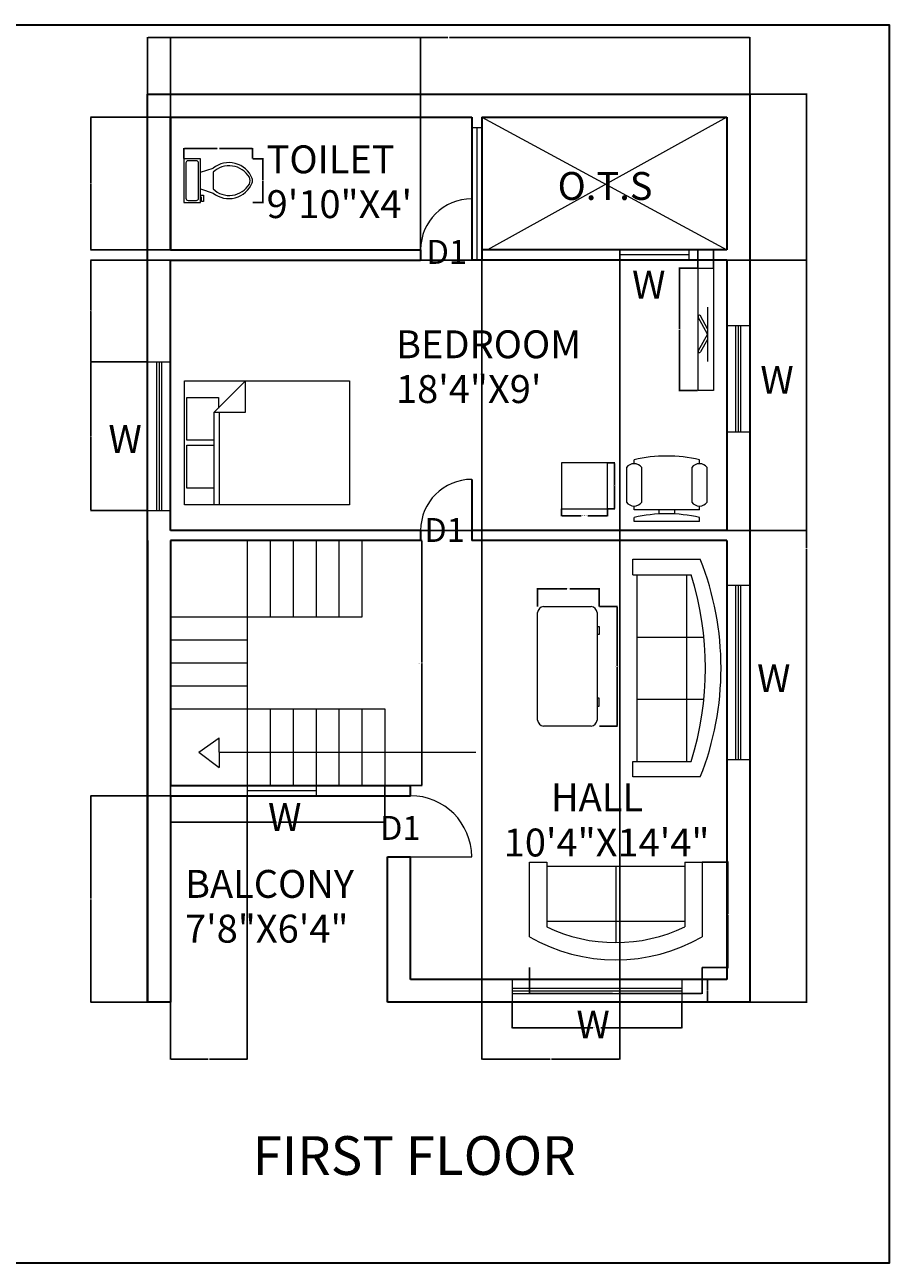
# Model space of a CAD drawing. Units: feet. Extents: x 38163 to 38841, y 65807 to 66292.
# Tile 3 of 3: x 38502 to 38841, y 65807 to 66292. Entities that reach past the tile are written whole.
import ezdxf

# ---------------------------------------------------------------- set-up
doc = ezdxf.new("R2010")
doc.units = ezdxf.units.FT
for name, color, linetype, lineweight in [('A-ANNO-DIMS', 2, 'Continuous', 18), ('A-ANNO-SYMB', 7, 'Continuous', 13), ('A-ANNO-TEXT', 7, 'Continuous', 18), ('A-ANNO-TITL', 7, 'Continuous', 25), ('A-ANNO-TTLB', 7, 'Continuous', 35), ('A-AREA-IDEN', 7, 'Continuous', 18), ('A-DOOR', 4, 'Continuous', 18), ('A-FLOR-FIXT', 9, 'Continuous', 18), ('A-FLOR-OPEN', 8, 'Continuous', 13), ('A-FLOR-STRS', 7, 'Continuous', 18), ('A-FURN', 8, 'Continuous', 18), ('A-GLAZ', 4, 'Continuous', 13), ('A-WALL', 7, 'Continuous', 35)]:
    doc.layers.add(name, color=color, linetype=linetype, lineweight=lineweight)
doc.styles.get("Standard").update_dxf_attribs({"font": 'arial.ttf'})
doc.dimstyles.get("Standard").update_dxf_attribs({"dimtxt": 0.18, "dimasz": 0.18, "dimexe": 0.18, "dimexo": 0.0625, "dimgap": 0.09, "dimtad": 0, "dimtih": 1, "dimtoh": 1, "dimdec": 4, "dimzin": 0, "dimdsep": 46, "dimtxsty": 'Standard', "dimcen": 0.09, "dimadec": 0, "dimazin": 0, "dimtfac": 1, "dimtdec": 4, "dimtofl": 0, "dimtmove": 0, "dimatfit": 3, "dimfxl": 1, "dimtolj": 1, "dimtzin": 0, "dimarcsym": 0})

# ---------------------------------------------------------------- blocks, each defined once
blk = doc.blocks.new('Toilet - top')
for p, q in [((9.5, -6), (9.5, -2)), ((-10, -8.5), (-8, -8.5)), ((-10, -9.5), (-10, -8.5)), ((-7, -9.5), (-10, -9.5)), ((-8, -8.5), (-8, -8)), ((-7, -8), (-7, -9.5)), ((-4, -8), (-6, -14)), ((4, -8), (6, -14)), ((4, -14), (-4, -14))]:
    blk.add_line(p, q)
blk.add_lwpolyline([(10.5, -8), (10.5, 0), (-10.5, 0), (-10.5, -8)], close=True)
for points in [[(-9.5, -2), (-9.5, -6)], [(8.5, -1), (-8.5, -1)], [(-8.5, -7), (8.5, -7)]]:
    blk.add_lwpolyline(points)
for centre, radius, start, end in [((-8.62, -1.88), 0.884, 81.8699, 188.1301), ((8.62, -1.88), 0.884, 351.8699, 98.1301), ((-8.62, -6.12), 0.884, 171.8699, 278.1301), ((8.62, -6.12), 0.884, 261.8699, 8.1301), ((3.52, -21.58), 12.17, 141.46911, 247.97143), ((4.2, -21.82), 11.33, 136.36773, 238.94682), ((-3.52, -21.58), 12.17, 292.02843, 38.53071), ((-4.2, -21.82), 11.33, 301.05301, 43.63209), ((0, -27.88), 4, 245.73182, 294.26817), ((0, -29), 4, 254.86053, 285.13947)]:
    blk.add_arc(centre, radius, start, end)
blk = doc.blocks.new('Bed - Queen')
for p, q in [((0, -80.00003), (0, 0)), ((0, 0), (59.99999, 0)), ((59.99999, 0), (59.99999, -80.00003)), ((7.99999, -1.2), (28.79998, -1.2)), ((7.99999, -14.4), (7.99999, -1.2)), ((28.79998, -1.2), (28.79998, -14.4)), ((31.19999, -1.2), (51.99999, -1.2)), ((31.19999, -14.4), (31.19999, -1.2)), ((51.99999, -1.2), (51.99999, -16.4)), ((0, -14.4), (44.8, -14.4)), ((44.8, -16.8), (0, -16.8)), ((59.99999, -29.6), (44.8, -14.4)), ((44.8, -14.4), (44.8, -29.6)), ((51.99999, -16.4), (46.79936, -16.4)), ((44.8, -29.6), (59.99999, -29.6)), ((59.99999, -80.00003), (0, -80.00003))]:
    blk.add_line(p, q)
blk = doc.blocks.new('Chair - Desk')
for p, q in [((-8.5, 0), (-8.5, -1)), ((-8.5, 0), (8.5, 0)), ((8.5, 0), (8.5, -1)), ((-8.5, -3), (-8.5, -4)), ((-8.5, -3), (8.5, -3)), ((-2, -3), (-2, -1.9355)), ((2, -1.9576), (2, -3)), ((8.5, -3), (8.5, -4)), ((-10.5, -5), (-10.5, -14)), ((-6.5, -14), (-6.5, -5)), ((6.5, -5), (6.5, -14)), ((10.5, -14), (10.5, -5)), ((-8.5, -15), (-8.5, -16)), ((8.5, -15), (8.5, -16))]:
    blk.add_line(p, q)
for centre, radius, start, end in [((0, 34.625), 36.625, 256.5803, 283.4197), ((-8.5, -6.5), 2.5, 36.8699, 143.1301), ((8.5, -6.5), 2.5, 36.8699, 143.1301), ((-8.5, -12.5), 2.5, 216.8699, 323.1301), ((0, 19.625), 36.625, 256.5803, 283.4197), ((8.5, -12.5), 2.5, 216.8699, 323.1301)]:
    blk.add_arc(centre, radius, start, end)
blk = doc.blocks.new('Desk - 30 x 60 in.')
for p, q in [((-26.999995, 0), (26.999995, 0)), ((-29.999995, -27), (-29.999995, -3)), ((29.999995, -3), (29.999995, -27)), ((26.999995, -30), (-26.999995, -30)), ((-20.000005, -30), (-20.000005, -31)), ((-20.000005, -31), (-16.000005, -31)), ((-16.000005, -31), (-16.000005, -30)), ((15.999995, -31), (15.999995, -30)), ((19.999995, -31), (15.999995, -31)), ((19.999995, -30), (19.999995, -31))]:
    blk.add_line(p, q)
for centre, start, end in [((-26.499995, -3.5), 98.1301, 171.8699), ((26.499995, -3.5), 8.130102, 81.8699), ((-26.499995, -26.5), 188.1301, 261.8699), ((26.499995, -26.5), 278.1301, 351.8699)]:
    blk.add_arc(centre, 3.535534, start, end)
blk = doc.blocks.new('Sofa - Roundback 7 ft.')
for p, q in [((-12.00002, -32.4421), (-12.00003, -6.5971)), ((11.99997, -32.4421), (11.99998, -6.5971)), ((-36.000027, -34), (-36.000027, -11.4696)), ((-35.999844, -13.3819), (35.9998, -13.3819)), ((35.99998, -34), (35.99998, -11.4696)), ((-36.000027, -32.4421), (35.99998, -32.4421))]:
    blk.add_line(p, q)
for points in [[(-36.000027, -34), (-42.000027, -34), (-42.000027, -8)], [(41.99998, -8), (41.99998, -34), (35.99998, -34)]]:
    blk.add_lwpolyline(points)
for centre, radius, start, end in [((0, -114.25), 114.25, 68.43141, 111.5686), ((-0.00001, -127.1968), 121.1968, 72.72033, 107.2797)]:
    blk.add_arc(centre, radius, start, end)
blk = doc.blocks.new('Sofa - Roundback Loveseat 5 ft.')
for p, q in [((0, -32.44198), (0, -5.99998)), ((-24, -33.99998), (-24, -11.46958)), ((24.00004, -33.99998), (24.00004, -11.46958)), ((-23.9998, -13.38178), (23.99986, -13.38178)), ((-24, -32.44198), (24.00004, -32.44198))]:
    blk.add_line(p, q)
for points in [[(-24, -33.99998), (-30, -33.99998), (-30, -7.99998)], [(30.00004, -7.99998), (30.00004, -33.99998), (24.00004, -33.99998)]]:
    blk.add_lwpolyline(points)
for centre, radius, start, end in [((0, -60.24998), 60.24998, 60.13715, 119.8628), ((0, -61.38438), 55.38444, 64.32083, 115.6792)]:
    blk.add_arc(centre, radius, start, end)
blk = doc.blocks.new('DOOR-SWING-24')
blk.add_line((0, 0), (24, 0))
blk.add_arc((0, 0), 24, 0, 90)
blk = doc.blocks.new('DOOR-SWING-20')
blk.add_line((20, 0), (20, 20))
blk.add_arc((20, 0), 20, 90, 180)
blk = doc.blocks.new('STAIR-HALF-TURN')
for p, q in [((30, 96), (30, 0)), ((39, 96), (39, 66)), ((48, 96), (48, 66)), ((57, 96), (57, 66)), ((66, 96), (66, 66)), ((75, 96), (75, 66)), ((75, 66), (0, 66)), ((30, 57), (0, 57)), ((30, 48), (0, 48)), ((30, 39), (0, 39)), ((0, 30), (84, 30)), ((39, 30), (39, 0)), ((48, 30), (48, 0)), ((57, 30), (57, 0)), ((66, 30), (66, 0)), ((75, 30), (75, 0)), ((84, 30), (84, 0))]:
    blk.add_line(p, q)
blk = doc.blocks.new('TABLE-SQUARE')
for p, q in [((18, 18), (0, 18)), ((0, 18), (0, 0)), ((18, 0), (18, 18)), ((0, 0), (18, 0))]:
    blk.add_line(p, q)
blk = doc.blocks.new('TV-CONSOLE')
for p, q in [((0.06, 48), (6.06, 48)), ((0.06, 0), (0.06, 48)), ((6.06, 48), (6.06, 0)), ((3.68, 24.21), (0.94, 29.3)), ((3.68, 32.75), (3.68, 11.44)), ((3.68, 22.09), (0.06, 28.83)), ((3.68, 22.09), (0.06, 15.67)), ((3.68, 20.06), (0.93, 15.18)), ((6.06, 0), (0.06, 0))]:
    blk.add_line(p, q)
for centre, start, end in [((0.5, 29.07), 28.2522, 208.2522), ((0.5, 15.42), 150.6168, 330.6168)]:
    blk.add_arc(centre, 0.5, start, end)
blk = doc.blocks.new('WIN-FRONT-HALL')
for p, q in [((0, 9), (0, 0)), ((0, 5.5), (66.57, 5.5)), ((66.57, 9), (66.57, 0)), ((0, 4.5), (66.57, 4.5)), ((0, 3.5), (66.57, 3.5))]:
    blk.add_line(p, q)
blk = doc.blocks.new('WIN-SIDE-HALL')
for p, q in [((0, 68.38), (9, 68.38)), ((3.5, 68.38), (3.5, 0)), ((4.5, 68.38), (4.5, 0)), ((5.5, 68.38), (5.5, 0)), ((0, 0), (9, 0))]:
    blk.add_line(p, q)
blk = doc.blocks.new('WIN-SIDE-REAR')
for p, q in [((0, 41.67), (9, 41.67)), ((3.5, 41.67), (3.5, 0)), ((4.5, 41.67), (4.5, 0)), ((5.5, 41.67), (5.5, 0)), ((0, 0), (9, 0))]:
    blk.add_line(p, q)
blk = doc.blocks.new('WIN-STAIR')
for p, q in [((0, 4), (0, 0)), ((0, 2), (27, 2)), ((27, 4), (27, 0))]:
    blk.add_line(p, q)
blk = doc.blocks.new('WIN-LIGHTWELL')
for p, q in [((0, 0), (0, 4)), ((0, 2), (27.16, 2)), ((27.16, 0), (27.16, 4))]:
    blk.add_line(p, q)
blk = doc.blocks.new('LIGHTWELL-CROSS')
for p, q in [((0, 52), (96, 0)), ((96, 52), (2.18, 0))]:
    blk.add_line(p, q)
blk = doc.blocks.new('STAIR-ARROWHEAD')
for p, q in [((0, 6), (8, 11.63)), ((8, 6), (8, 11.63)), ((0, 6), (8, 0)), ((8, 6), (8, 0)), ((8, 0), (8, 0))]:
    blk.add_line(p, q)
blk = doc.blocks.new('*D29')
at = {"layer": 'A-ANNO-DIMS', "color": 0, "lineweight": -2, "transparency": 16777216}
for p, q in [((38727.19, 66064.14), (38734.33, 66064.14)), ((38734.15, 66063.96), (38734.15, 66040.91)), ((38734.15, 66017.51), (38734.15, 66040.55)), ((38727.19, 66017.33), (38734.33, 66017.33))]:
    blk.add_line(p, q, dxfattribs=at)
at = {"layer": 'A-ANNO-DIMS', "color": 0, "transparency": 16777216}
for points in [[(38734.12, 66063.96), (38734.18, 66063.96), (38734.15, 66064.14)], [(38734.12, 66017.51), (38734.18, 66017.51), (38734.15, 66017.33)]]:
    blk.add_solid(points, dxfattribs=at)
at = {"layer": 'Defpoints', "color": 0, "transparency": 16777216}
for p in [(38727.13, 66064.14), (38734.15, 66064.14), (38727.13, 66017.33)]:
    blk.add_point(p, dxfattribs=at)
at = {"layer": 'A-ANNO-DIMS', "color": 0, "transparency": 16777216, "insert": (38734.15, 66040.73), "char_height": 0.18, "attachment_point": 5}
blk.add_mtext('\\A1;DESK 47 TYP.', dxfattribs=at)
blk = doc.blocks.new('*D30')
at = {"layer": 'A-ANNO-DIMS', "color": 0, "lineweight": -2, "transparency": 16777216}
for p, q in [((38702.94, 66064.2), (38702.94, 66071.34)), ((38703.12, 66071.16), (38714.51, 66071.16)), ((38726.95, 66071.16), (38715.57, 66071.16)), ((38727.13, 66064.2), (38727.13, 66071.34))]:
    blk.add_line(p, q, dxfattribs=at)
at = {"layer": 'A-ANNO-DIMS', "color": 0, "transparency": 16777216}
for points in [[(38703.12, 66071.19), (38703.12, 66071.13), (38702.94, 66071.16)], [(38726.95, 66071.19), (38726.95, 66071.13), (38727.13, 66071.16)]]:
    blk.add_solid(points, dxfattribs=at)
at = {"layer": 'Defpoints', "color": 0, "transparency": 16777216}
for p in [(38702.94, 66071.16), (38702.94, 66064.14), (38727.13, 66064.14)]:
    blk.add_point(p, dxfattribs=at)
at = {"layer": 'A-ANNO-DIMS', "color": 0, "transparency": 16777216, "insert": (38715.04, 66071.16), "char_height": 0.18, "attachment_point": 5}
blk.add_mtext('\\A1;24 TYP.', dxfattribs=at)
blk = doc.blocks.new('*D33')
at = {"layer": 'A-ANNO-DIMS', "color": 0, "lineweight": -2, "transparency": 16777216}
for p, q in [((38699.8, 65922.6), (38699.8, 65912.34)), ((38767.45, 65922.6), (38767.45, 65912.34)), ((38699.98, 65912.52), (38732.4, 65912.52)), ((38767.27, 65912.52), (38734.85, 65912.52))]:
    blk.add_line(p, q, dxfattribs=at)
at = {"layer": 'A-ANNO-DIMS', "color": 0, "transparency": 16777216}
for points in [[(38699.98, 65912.55), (38699.98, 65912.49), (38699.8, 65912.52)], [(38767.27, 65912.55), (38767.27, 65912.49), (38767.45, 65912.52)]]:
    blk.add_solid(points, dxfattribs=at)
at = {"layer": 'Defpoints', "color": 0, "transparency": 16777216}
for p in [(38699.8, 65922.66), (38767.45, 65922.66), (38699.8, 65912.52)]:
    blk.add_point(p, dxfattribs=at)
at = {"layer": 'A-ANNO-DIMS', "color": 0, "transparency": 16777216, "insert": (38733.63, 65912.52), "char_height": 0.18, "attachment_point": 5}
blk.add_mtext('\\A1;LOVESEAT 68 TYP.', dxfattribs=at)
blk = doc.blocks.new('*D34')
at = {"layer": 'A-ANNO-DIMS', "color": 0, "lineweight": -2, "transparency": 16777216}
for p, q in [((38767.51, 65964.01), (38777.78, 65964.01)), ((38777.6, 65963.83), (38777.6, 65943.52)), ((38777.6, 65922.84), (38777.6, 65943.16)), ((38767.51, 65922.66), (38777.78, 65922.66))]:
    blk.add_line(p, q, dxfattribs=at)
at = {"layer": 'A-ANNO-DIMS', "color": 0, "transparency": 16777216}
for points in [[(38777.57, 65963.83), (38777.63, 65963.83), (38777.6, 65964.01)], [(38777.57, 65922.84), (38777.63, 65922.84), (38777.6, 65922.66)]]:
    blk.add_solid(points, dxfattribs=at)
at = {"layer": 'Defpoints', "color": 0, "transparency": 16777216}
for p in [(38767.45, 65964.01), (38767.45, 65922.66), (38777.6, 65922.66)]:
    blk.add_point(p, dxfattribs=at)
at = {"layer": 'A-ANNO-DIMS', "color": 0, "transparency": 16777216, "insert": (38777.6, 65943.34), "char_height": 0.18, "attachment_point": 5}
blk.add_mtext('\\A1;41 TYP.', dxfattribs=at)
blk = doc.blocks.new('*D35')
at = {"layer": 'A-ANNO-DIMS', "color": 0, "lineweight": -2, "transparency": 16777216}
for p, q in [((38643.22, 66090.01), (38657.74, 66090.01)), ((38657.56, 66089.83), (38657.56, 66042.2)), ((38657.56, 65994.19), (38657.56, 66041.83)), ((38643.22, 65994.01), (38657.74, 65994.01))]:
    blk.add_line(p, q, dxfattribs=at)
at = {"layer": 'A-ANNO-DIMS', "color": 0, "transparency": 16777216}
for points in [[(38657.53, 66089.83), (38657.59, 66089.83), (38657.56, 66090.01)], [(38657.53, 65994.19), (38657.59, 65994.19), (38657.56, 65994.01)]]:
    blk.add_solid(points, dxfattribs=at)
at = {"layer": 'Defpoints', "color": 0, "transparency": 16777216}
for p in [(38643.16, 66090.01), (38657.56, 66090.01), (38643.16, 65994.01)]:
    blk.add_point(p, dxfattribs=at)
at = {"layer": 'A-ANNO-DIMS', "color": 0, "transparency": 16777216, "insert": (38657.56, 66042.01), "char_height": 0.18, "attachment_point": 5}
blk.add_mtext('\\A1;HALF-TURN STAIR 96 TYP.', dxfattribs=at)
blk = doc.blocks.new('*D36')
at = {"layer": 'A-ANNO-DIMS', "color": 0, "lineweight": -2, "transparency": 16777216}
for p, q in [((38559.16, 65993.95), (38559.16, 65979.43)), ((38643.16, 65993.95), (38643.16, 65979.43)), ((38559.34, 65979.61), (38600.63, 65979.61)), ((38642.98, 65979.61), (38601.69, 65979.61))]:
    blk.add_line(p, q, dxfattribs=at)
at = {"layer": 'A-ANNO-DIMS', "color": 0, "transparency": 16777216}
for points in [[(38559.34, 65979.64), (38559.34, 65979.58), (38559.16, 65979.61)], [(38642.98, 65979.64), (38642.98, 65979.58), (38643.16, 65979.61)]]:
    blk.add_solid(points, dxfattribs=at)
at = {"layer": 'Defpoints', "color": 0, "transparency": 16777216}
for p in [(38559.16, 65994.01), (38643.16, 65994.01), (38643.16, 65979.61)]:
    blk.add_point(p, dxfattribs=at)
at = {"layer": 'A-ANNO-DIMS', "color": 0, "transparency": 16777216, "insert": (38601.16, 65979.61), "char_height": 0.18, "attachment_point": 5}
blk.add_mtext('\\A1;84 TYP.', dxfattribs=at)
blk = doc.blocks.new('*D37')
at = {"layer": 'A-ANNO-DIMS', "color": 0, "lineweight": -2, "transparency": 16777216}
for p, q in [((38712.38, 66102.41), (38712.38, 66099.6)), ((38730.38, 66102.41), (38730.38, 66099.6)), ((38712.56, 66099.78), (38720.09, 66099.78)), ((38730.2, 66099.78), (38722.67, 66099.78))]:
    blk.add_line(p, q, dxfattribs=at)
at = {"layer": 'A-ANNO-DIMS', "color": 0, "transparency": 16777216}
for points in [[(38712.56, 66099.81), (38712.56, 66099.75), (38712.38, 66099.78)], [(38730.2, 66099.81), (38730.2, 66099.75), (38730.38, 66099.78)]]:
    blk.add_solid(points, dxfattribs=at)
at = {"layer": 'Defpoints', "color": 0, "transparency": 16777216}
for p in [(38712.38, 66102.48), (38730.38, 66102.48), (38730.38, 66099.78)]:
    blk.add_point(p, dxfattribs=at)
at = {"layer": 'A-ANNO-DIMS', "color": 0, "transparency": 16777216, "insert": (38721.38, 66099.78), "char_height": 0.18, "attachment_point": 5}
blk.add_mtext('\\A1;SIDE TABLE 18 TYP.', dxfattribs=at)
blk = doc.blocks.new('*D38')
at = {"layer": 'A-ANNO-DIMS', "color": 0, "lineweight": -2, "transparency": 16777216}
for p, q in [((38730.44, 66120.48), (38733.26, 66120.48)), ((38733.08, 66120.3), (38733.08, 66111.66)), ((38733.08, 66102.66), (38733.08, 66111.3)), ((38730.44, 66102.48), (38733.26, 66102.48))]:
    blk.add_line(p, q, dxfattribs=at)
at = {"layer": 'A-ANNO-DIMS', "color": 0, "transparency": 16777216}
for points in [[(38733.05, 66120.3), (38733.11, 66120.3), (38733.08, 66120.48)], [(38733.05, 66102.66), (38733.11, 66102.66), (38733.08, 66102.48)]]:
    blk.add_solid(points, dxfattribs=at)
at = {"layer": 'Defpoints', "color": 0, "transparency": 16777216}
for p in [(38730.38, 66120.48), (38733.08, 66120.48), (38730.38, 66102.48)]:
    blk.add_point(p, dxfattribs=at)
at = {"layer": 'A-ANNO-DIMS', "color": 0, "transparency": 16777216, "insert": (38733.08, 66111.48), "char_height": 0.18, "attachment_point": 5}
blk.add_mtext('\\A1;18 TYP.', dxfattribs=at)
blk = doc.blocks.new('*D39')
at = {"layer": 'A-ANNO-DIMS', "color": 0, "lineweight": -2, "transparency": 16777216}
for p, q in [((38765.71, 66196.8), (38758.39, 66196.8)), ((38758.57, 66196.62), (38758.57, 66172.99)), ((38758.57, 66148.98), (38758.57, 66172.62)), ((38765.71, 66148.8), (38758.39, 66148.8))]:
    blk.add_line(p, q, dxfattribs=at)
at = {"layer": 'A-ANNO-DIMS', "color": 0, "transparency": 16777216}
for points in [[(38758.54, 66196.62), (38758.6, 66196.62), (38758.57, 66196.8)], [(38758.54, 66148.98), (38758.6, 66148.98), (38758.57, 66148.8)]]:
    blk.add_solid(points, dxfattribs=at)
at = {"layer": 'Defpoints', "color": 0, "transparency": 16777216}
for p in [(38758.57, 66196.8), (38765.77, 66196.8), (38765.77, 66148.8)]:
    blk.add_point(p, dxfattribs=at)
at = {"layer": 'A-ANNO-DIMS', "color": 0, "transparency": 16777216, "insert": (38758.57, 66172.8), "char_height": 0.18, "attachment_point": 5}
blk.add_mtext('\\A1;TV CONSOLE 48 TYP.', dxfattribs=at)
blk = doc.blocks.new('*D40')
at = {"layer": 'A-ANNO-DIMS', "color": 0, "lineweight": -2, "transparency": 16777216}
for p, q in [((38765.77, 66196.87), (38765.77, 66204.18)), ((38765.95, 66204), (38768.38, 66204)), ((38771.72, 66204), (38769.29, 66204)), ((38771.9, 66196.87), (38771.9, 66204.18))]:
    blk.add_line(p, q, dxfattribs=at)
at = {"layer": 'A-ANNO-DIMS', "color": 0, "transparency": 16777216}
for points in [[(38765.95, 66204.03), (38765.95, 66203.97), (38765.77, 66204)], [(38771.72, 66204.03), (38771.72, 66203.97), (38771.9, 66204)]]:
    blk.add_solid(points, dxfattribs=at)
at = {"layer": 'Defpoints', "color": 0, "transparency": 16777216}
for p in [(38771.9, 66204), (38765.77, 66196.8), (38771.9, 66196.8)]:
    blk.add_point(p, dxfattribs=at)
at = {"layer": 'A-ANNO-DIMS', "color": 0, "transparency": 16777216, "insert": (38768.84, 66204), "char_height": 0.18, "attachment_point": 5}
blk.add_mtext('\\A1;6 TYP.', dxfattribs=at)
blk = doc.blocks.new('*D41')
at = {"layer": 'A-ANNO-DIMS', "color": 0, "lineweight": -2, "transparency": 16777216}
for p, q in [((38692.96, 65908.95), (38692.96, 65898.85)), ((38759.53, 65908.95), (38759.53, 65898.85)), ((38693.14, 65899.03), (38724.67, 65899.03)), ((38759.35, 65899.03), (38727.82, 65899.03))]:
    blk.add_line(p, q, dxfattribs=at)
at = {"layer": 'A-ANNO-DIMS', "color": 0, "transparency": 16777216}
for points in [[(38693.14, 65899.06), (38693.14, 65899), (38692.96, 65899.03)], [(38759.35, 65899.06), (38759.35, 65899), (38759.53, 65899.03)]]:
    blk.add_solid(points, dxfattribs=at)
at = {"layer": 'Defpoints', "color": 0, "transparency": 16777216}
for p in [(38692.96, 65909.01), (38759.53, 65909.01), (38759.53, 65899.03)]:
    blk.add_point(p, dxfattribs=at)
at = {"layer": 'A-ANNO-DIMS', "color": 0, "transparency": 16777216, "insert": (38726.24, 65899.03), "char_height": 0.18, "attachment_point": 5}
blk.add_mtext('\\A1;FRONT WINDOW 67 TYP.', dxfattribs=at)
blk = doc.blocks.new('*D42')
at = {"layer": 'A-ANNO-DIMS', "color": 0, "lineweight": -2, "transparency": 16777216}
for p, q in [((38759.59, 65918.01), (38769.69, 65918.01)), ((38769.51, 65917.83), (38769.51, 65913.69)), ((38769.51, 65909.19), (38769.51, 65913.33)), ((38759.59, 65909.01), (38769.69, 65909.01))]:
    blk.add_line(p, q, dxfattribs=at)
at = {"layer": 'A-ANNO-DIMS', "color": 0, "transparency": 16777216}
for points in [[(38769.48, 65917.83), (38769.54, 65917.83), (38769.51, 65918.01)], [(38769.48, 65909.19), (38769.54, 65909.19), (38769.51, 65909.01)]]:
    blk.add_solid(points, dxfattribs=at)
at = {"layer": 'Defpoints', "color": 0, "transparency": 16777216}
for p in [(38759.53, 65918.01), (38769.51, 65918.01), (38759.53, 65909.01)]:
    blk.add_point(p, dxfattribs=at)
at = {"layer": 'A-ANNO-DIMS', "color": 0, "transparency": 16777216, "insert": (38769.51, 65913.51), "char_height": 0.18, "attachment_point": 5}
blk.add_mtext('\\A1;9 TYP.', dxfattribs=at)
blk = doc.blocks.new('*D51')
at = {"layer": 'A-ANNO-DIMS', "color": 0, "lineweight": -2, "transparency": 16777216}
for p, q in [((38564.38, 66239.76), (38564.38, 66243.91)), ((38564.56, 66243.73), (38577.37, 66243.73)), ((38591.12, 66243.73), (38578.31, 66243.73)), ((38591.3, 66239.76), (38591.3, 66243.91))]:
    blk.add_line(p, q, dxfattribs=at)
at = {"layer": 'A-ANNO-DIMS', "color": 0, "transparency": 16777216}
for points in [[(38564.56, 66243.76), (38564.56, 66243.7), (38564.38, 66243.73)], [(38591.12, 66243.76), (38591.12, 66243.7), (38591.3, 66243.73)]]:
    blk.add_solid(points, dxfattribs=at)
at = {"layer": 'Defpoints', "color": 0, "transparency": 16777216}
for p in [(38564.38, 66243.73), (38564.38, 66239.69), (38591.3, 66239.69)]:
    blk.add_point(p, dxfattribs=at)
at = {"layer": 'A-ANNO-DIMS', "color": 0, "transparency": 16777216, "insert": (38577.84, 66243.73), "char_height": 0.18, "attachment_point": 5}
blk.add_mtext('\\A1;WC 27', dxfattribs=at)
blk = doc.blocks.new('*D52')
at = {"layer": 'A-ANNO-DIMS', "color": 0, "lineweight": -2, "transparency": 16777216}
for p, q in [((38591.36, 66239.69), (38595.52, 66239.69)), ((38595.34, 66239.51), (38595.34, 66231.32)), ((38595.34, 66222.77), (38595.34, 66230.96)), ((38591.36, 66222.59), (38595.52, 66222.59))]:
    blk.add_line(p, q, dxfattribs=at)
at = {"layer": 'A-ANNO-DIMS', "color": 0, "transparency": 16777216}
for points in [[(38595.31, 66239.51), (38595.37, 66239.51), (38595.34, 66239.69)], [(38595.31, 66222.77), (38595.37, 66222.77), (38595.34, 66222.59)]]:
    blk.add_solid(points, dxfattribs=at)
at = {"layer": 'Defpoints', "color": 0, "transparency": 16777216}
for p in [(38591.3, 66239.69), (38595.34, 66239.69), (38591.3, 66222.59)]:
    blk.add_point(p, dxfattribs=at)
at = {"layer": 'A-ANNO-DIMS', "color": 0, "transparency": 16777216, "insert": (38595.34, 66231.14), "char_height": 0.18, "attachment_point": 5}
blk.add_mtext('\\A1;17', dxfattribs=at)
blk = doc.blocks.new('*D59')
at = {"layer": 'A-ANNO-DIMS', "color": 0, "lineweight": -2, "transparency": 16777216}
for p, q in [((38550.16, 66265.08), (38550.16, 66287.44)), ((38550.34, 66287.26), (38667.87, 66287.26)), ((38785.98, 66287.26), (38668.45, 66287.26)), ((38786.16, 66265.08), (38786.16, 66287.44))]:
    blk.add_line(p, q, dxfattribs=at)
at = {"layer": 'A-ANNO-DIMS', "color": 0, "transparency": 16777216}
for points in [[(38550.34, 66287.29), (38550.34, 66287.23), (38550.16, 66287.26)], [(38785.98, 66287.29), (38785.98, 66287.23), (38786.16, 66287.26)]]:
    blk.add_solid(points, dxfattribs=at)
at = {"layer": 'Defpoints', "color": 0, "transparency": 16777216}
for p in [(38786.16, 66287.26), (38550.16, 66265.01), (38786.16, 66265.01)]:
    blk.add_point(p, dxfattribs=at)
at = {"layer": 'A-ANNO-DIMS', "color": 0, "transparency": 16777216, "insert": (38668.16, 66287.26), "char_height": 0.18, "attachment_point": 5}
blk.add_mtext('\\A1;236', dxfattribs=at)
blk = doc.blocks.new('*D60')
at = {"layer": 'A-ANNO-DIMS', "color": 0, "lineweight": -2, "transparency": 16777216}
for p, q in [((38786.22, 66265.01), (38808.59, 66265.01)), ((38808.41, 66264.83), (38808.41, 66087.19)), ((38808.41, 65909.19), (38808.41, 66086.83)), ((38786.22, 65909.01), (38808.59, 65909.01))]:
    blk.add_line(p, q, dxfattribs=at)
at = {"layer": 'A-ANNO-DIMS', "color": 0, "transparency": 16777216}
for points in [[(38808.38, 66264.83), (38808.44, 66264.83), (38808.41, 66265.01)], [(38808.38, 65909.19), (38808.44, 65909.19), (38808.41, 65909.01)]]:
    blk.add_solid(points, dxfattribs=at)
at = {"layer": 'Defpoints', "color": 0, "transparency": 16777216}
for p in [(38786.16, 66265.01), (38808.41, 66265.01), (38786.16, 65909.01)]:
    blk.add_point(p, dxfattribs=at)
at = {"layer": 'A-ANNO-DIMS', "color": 0, "transparency": 16777216, "insert": (38808.41, 66087.01), "char_height": 0.18, "attachment_point": 5}
blk.add_mtext('\\A1;356', dxfattribs=at)
blk = doc.blocks.new('*D66')
at = {"layer": 'A-ANNO-DIMS', "color": 0, "lineweight": -2, "transparency": 16777216}
for p, q in [((38559.1, 66200.01), (38527.73, 66200.01)), ((38527.91, 66199.83), (38527.91, 66180.22)), ((38527.91, 66160.24), (38527.91, 66179.85)), ((38550.1, 66160.06), (38527.73, 66160.06))]:
    blk.add_line(p, q, dxfattribs=at)
at = {"layer": 'A-ANNO-DIMS', "color": 0, "transparency": 16777216}
for points in [[(38527.88, 66199.83), (38527.94, 66199.83), (38527.91, 66200.01)], [(38527.88, 66160.24), (38527.94, 66160.24), (38527.91, 66160.06)]]:
    blk.add_solid(points, dxfattribs=at)
at = {"layer": 'Defpoints', "color": 0, "transparency": 16777216}
for p in [(38527.91, 66200.01), (38559.16, 66200.01), (38550.16, 66160.06)]:
    blk.add_point(p, dxfattribs=at)
at = {"layer": 'A-ANNO-DIMS', "color": 0, "transparency": 16777216, "insert": (38527.91, 66180.04), "char_height": 0.18, "attachment_point": 5}
blk.add_mtext('\\A1;39.95', dxfattribs=at)
blk = doc.blocks.new('*D67')
at = {"layer": 'A-ANNO-DIMS', "color": 0, "lineweight": -2, "transparency": 16777216}
for p, q in [((38550.1, 66160.06), (38527.73, 66160.06)), ((38527.91, 66159.88), (38527.91, 66131.15)), ((38527.91, 66102.05), (38527.91, 66130.78)), ((38550.1, 66101.87), (38527.73, 66101.87))]:
    blk.add_line(p, q, dxfattribs=at)
at = {"layer": 'A-ANNO-DIMS', "color": 0, "transparency": 16777216}
for points in [[(38527.88, 66159.88), (38527.94, 66159.88), (38527.91, 66160.06)], [(38527.88, 66102.05), (38527.94, 66102.05), (38527.91, 66101.87)]]:
    blk.add_solid(points, dxfattribs=at)
at = {"layer": 'Defpoints', "color": 0, "transparency": 16777216}
for p in [(38527.91, 66160.06), (38550.16, 66160.06), (38550.16, 66101.87)]:
    blk.add_point(p, dxfattribs=at)
at = {"layer": 'A-ANNO-DIMS', "color": 0, "transparency": 16777216, "insert": (38527.91, 66130.96), "char_height": 0.18, "attachment_point": 5}
blk.add_mtext('\\A1;58.2', dxfattribs=at)
blk = doc.blocks.new('*D70')
at = {"layer": 'A-ANNO-DIMS', "color": 0, "lineweight": -2, "transparency": 16777216}
for p, q in [((38681.16, 66203.95), (38681.16, 65886.58)), ((38735.16, 66203.95), (38735.16, 65886.58)), ((38681.34, 65886.76), (38707.94, 65886.76)), ((38734.98, 65886.76), (38708.38, 65886.76))]:
    blk.add_line(p, q, dxfattribs=at)
at = {"layer": 'A-ANNO-DIMS', "color": 0, "transparency": 16777216}
for points in [[(38681.34, 65886.79), (38681.34, 65886.73), (38681.16, 65886.76)], [(38734.98, 65886.79), (38734.98, 65886.73), (38735.16, 65886.76)]]:
    blk.add_solid(points, dxfattribs=at)
at = {"layer": 'Defpoints', "color": 0, "transparency": 16777216}
for p in [(38681.16, 66204.01), (38735.16, 66204.01), (38735.16, 65886.76)]:
    blk.add_point(p, dxfattribs=at)
at = {"layer": 'A-ANNO-DIMS', "color": 0, "transparency": 16777216, "insert": (38708.16, 65886.76), "char_height": 0.18, "attachment_point": 5}
blk.add_mtext('\\A1;54', dxfattribs=at)
blk = doc.blocks.new('*D71')
at = {"layer": 'A-ANNO-DIMS', "color": 0, "lineweight": -2, "transparency": 16777216}
for p, q in [((38559.16, 65989.95), (38559.16, 65886.58)), ((38589.16, 65989.95), (38589.16, 65886.58)), ((38559.34, 65886.76), (38573.94, 65886.76)), ((38588.98, 65886.76), (38574.38, 65886.76))]:
    blk.add_line(p, q, dxfattribs=at)
at = {"layer": 'A-ANNO-DIMS', "color": 0, "transparency": 16777216}
for points in [[(38559.34, 65886.79), (38559.34, 65886.73), (38559.16, 65886.76)], [(38588.98, 65886.79), (38588.98, 65886.73), (38589.16, 65886.76)]]:
    blk.add_solid(points, dxfattribs=at)
at = {"layer": 'Defpoints', "color": 0, "transparency": 16777216}
for p in [(38559.16, 65990.01), (38589.16, 65990.01), (38589.16, 65886.76)]:
    blk.add_point(p, dxfattribs=at)
at = {"layer": 'A-ANNO-DIMS', "color": 0, "transparency": 16777216, "insert": (38574.16, 65886.76), "char_height": 0.18, "attachment_point": 5}
blk.add_mtext('\\A1;30', dxfattribs=at)
blk = doc.blocks.new('*D72')
at = {"layer": 'A-ANNO-DIMS', "color": 0, "lineweight": -2, "transparency": 16777216}
for p, q in [((38559.16, 66204.08), (38559.16, 66287.44)), ((38559.34, 66287.26), (38607.94, 66287.26)), ((38656.98, 66287.26), (38608.38, 66287.26)), ((38657.16, 66204.08), (38657.16, 66287.44))]:
    blk.add_line(p, q, dxfattribs=at)
at = {"layer": 'A-ANNO-DIMS', "color": 0, "transparency": 16777216}
for points in [[(38559.34, 66287.29), (38559.34, 66287.23), (38559.16, 66287.26)], [(38656.98, 66287.29), (38656.98, 66287.23), (38657.16, 66287.26)]]:
    blk.add_solid(points, dxfattribs=at)
at = {"layer": 'Defpoints', "color": 0, "transparency": 16777216}
for p in [(38657.16, 66287.26), (38559.16, 66204.01), (38657.16, 66204.01)]:
    blk.add_point(p, dxfattribs=at)
at = {"layer": 'A-ANNO-DIMS', "color": 0, "transparency": 16777216, "insert": (38608.16, 66287.26), "char_height": 0.18, "attachment_point": 5}
blk.add_mtext('\\A1;98', dxfattribs=at)
blk = doc.blocks.new('*D77')
at = {"layer": 'A-ANNO-DIMS', "color": 0, "lineweight": -2, "transparency": 16777216}
for p, q in [((38559.1, 65990.01), (38527.73, 65990.01)), ((38527.91, 65989.83), (38527.91, 65949.69)), ((38527.91, 65909.19), (38527.91, 65949.33)), ((38559.1, 65909.01), (38527.73, 65909.01))]:
    blk.add_line(p, q, dxfattribs=at)
at = {"layer": 'A-ANNO-DIMS', "color": 0, "transparency": 16777216}
for points in [[(38527.88, 65989.83), (38527.94, 65989.83), (38527.91, 65990.01)], [(38527.88, 65909.19), (38527.94, 65909.19), (38527.91, 65909.01)]]:
    blk.add_solid(points, dxfattribs=at)
at = {"layer": 'Defpoints', "color": 0, "transparency": 16777216}
for p in [(38527.91, 65990.01), (38559.16, 65990.01), (38559.16, 65909.01)]:
    blk.add_point(p, dxfattribs=at)
at = {"layer": 'A-ANNO-DIMS', "color": 0, "transparency": 16777216, "insert": (38527.91, 65949.51), "char_height": 0.18, "attachment_point": 5}
blk.add_mtext('\\A1;81', dxfattribs=at)
blk = doc.blocks.new('*D78')
at = {"layer": 'A-ANNO-DIMS', "color": 0, "lineweight": -2, "transparency": 16777216}
for p, q in [((38559.22, 66200.01), (38808.59, 66200.01)), ((38808.41, 66199.83), (38808.41, 66147.19)), ((38808.41, 66094.19), (38808.41, 66146.83)), ((38559.22, 66094.01), (38808.59, 66094.01))]:
    blk.add_line(p, q, dxfattribs=at)
at = {"layer": 'A-ANNO-DIMS', "color": 0, "transparency": 16777216}
for points in [[(38808.38, 66199.83), (38808.44, 66199.83), (38808.41, 66200.01)], [(38808.38, 66094.19), (38808.44, 66094.19), (38808.41, 66094.01)]]:
    blk.add_solid(points, dxfattribs=at)
at = {"layer": 'Defpoints', "color": 0, "transparency": 16777216}
for p in [(38559.16, 66200.01), (38808.41, 66200.01), (38559.16, 66094.01)]:
    blk.add_point(p, dxfattribs=at)
at = {"layer": 'A-ANNO-DIMS', "color": 0, "transparency": 16777216, "insert": (38808.41, 66147.01), "char_height": 0.18, "attachment_point": 5}
blk.add_mtext('\\A1;106', dxfattribs=at)
blk = doc.blocks.new('*D79')
at = {"layer": 'A-ANNO-DIMS', "color": 0, "lineweight": -2, "transparency": 16777216}
for p, q in [((38559.1, 66256.01), (38527.73, 66256.01)), ((38527.91, 66255.83), (38527.91, 66230.19)), ((38527.91, 66204.19), (38527.91, 66229.83)), ((38559.1, 66204.01), (38527.73, 66204.01))]:
    blk.add_line(p, q, dxfattribs=at)
at = {"layer": 'A-ANNO-DIMS', "color": 0, "transparency": 16777216}
for points in [[(38527.88, 66255.83), (38527.94, 66255.83), (38527.91, 66256.01)], [(38527.88, 66204.19), (38527.94, 66204.19), (38527.91, 66204.01)]]:
    blk.add_solid(points, dxfattribs=at)
at = {"layer": 'Defpoints', "color": 0, "transparency": 16777216}
for p in [(38527.91, 66256.01), (38559.16, 66256.01), (38559.16, 66204.01)]:
    blk.add_point(p, dxfattribs=at)
at = {"layer": 'A-ANNO-DIMS', "color": 0, "transparency": 16777216, "insert": (38527.91, 66230.01), "char_height": 0.18, "attachment_point": 5}
blk.add_mtext('\\A1;52', dxfattribs=at)

msp = doc.modelspace()

# ---------------------------------------------------------------- linework, layer by layer
at = {"layer": 'A-ANNO-SYMB'}
msp.add_line((38578.203, 66007.084), (38678.782, 66007.084), dxfattribs=at)
at = {"layer": 'A-ANNO-TTLB'}
msp.add_lwpolyline([(38163.261, 66292.238), (38840.784, 66292.238), (38840.784, 65806.731), (38163.261, 65806.731)], close=True, dxfattribs=at)
at = {"layer": 'A-GLAZ'}
for p, q in [((38677.16, 66252.001), (38681.16, 66252.001)), ((38679.16, 66252.001), (38679.16, 66200.013)), ((38550.16, 66160.061), (38559.16, 66160.061)), ((38553.66, 66160.061), (38553.66, 66101.866)), ((38554.66, 66160.061), (38554.66, 66101.866)), ((38555.66, 66160.061), (38555.66, 66101.866)), ((38550.16, 66101.866), (38559.16, 66101.866))]:
    msp.add_line(p, q, dxfattribs=at)
at = {"layer": 'A-WALL'}
for p, q in [((38550.16, 66265.013), (38786.16, 66265.013)), ((38550.16, 65909.013), (38550.16, 66265.013)), ((38681.16, 66265.013), (38786.16, 66265.013)), ((38786.16, 66265.013), (38786.16, 65909.013)), ((38559.16, 66256.013), (38677.16, 66256.013)), ((38559.16, 66256.013), (38559.16, 66204.013)), ((38559.16, 66204.013), (38559.16, 66256.013)), ((38677.16, 66256.013), (38677.16, 66212.078)), ((38681.16, 66256.013), (38681.16, 66204.013)), ((38681.16, 66256.013), (38777.16, 66256.013)), ((38777.16, 66256.013), (38777.16, 66204.013)), ((38677.16, 66212.078), (38677.16, 66200.013)), ((38559.16, 66204.013), (38657.16, 66204.013)), ((38657.16, 66204.013), (38657.16, 66200.013)), ((38693.16, 66204.013), (38681.16, 66204.013)), ((38681.16, 66204.013), (38681.16, 66200.013)), ((38777.16, 66204.013), (38693.16, 66204.013)), ((38559.16, 66094.013), (38559.16, 66200.013)), ((38559.16, 66200.013), (38657.16, 66200.013)), ((38777.16, 66200.013), (38677.16, 66200.013)), ((38777.16, 66200.013), (38777.16, 66094.013)), ((38786.16, 66200.013), (38786.16, 66094.013)), ((38677.16, 66114.013), (38677.16, 66090.013)), ((38657.16, 66094.013), (38559.16, 66094.013)), ((38657.16, 66094.013), (38657.16, 66090.013)), ((38777.16, 66094.013), (38677.16, 66094.013)), ((38550.16, 66090.013), (38550.16, 65909.013)), ((38657.16, 66090.013), (38559.16, 66090.013)), ((38657.16, 66090.013), (38559.16, 66090.013)), ((38559.16, 66090.013), (38559.16, 65994.013)), ((38777.16, 66090.013), (38677.16, 66090.013)), ((38681.16, 66090.013), (38677.16, 66090.013)), ((38777.16, 66090.013), (38777.16, 65918.013)), ((38777.16, 66090.013), (38777.16, 66071.969)), ((38786.16, 66090.013), (38786.16, 65909.013)), ((38559.16, 65994.013), (38653.16, 65994.013)), ((38653.16, 65990.013), (38653.16, 65994.013)), ((38559.16, 65990.013), (38653.16, 65990.013)), ((38559.16, 65990.013), (38559.16, 65909.013)), ((38644.16, 65909.013), (38644.16, 65966.013)), ((38644.16, 65966.013), (38653.16, 65966.013)), ((38653.16, 65918.013), (38653.16, 65966.013)), ((38777.16, 65918.013), (38653.16, 65918.013)), ((38559.16, 65909.013), (38550.16, 65909.013)), ((38786.16, 65909.013), (38644.16, 65909.013))]:
    msp.add_line(p, q, dxfattribs=at)

# ---------------------------------------------------------------- block references
at = {"layer": 'A-ANNO-SYMB'}
msp.add_blockref('STAIR-ARROWHEAD', (38570.203, 66001.084), dxfattribs=at)
at = {"layer": 'A-DOOR'}
for name, p in [('DOOR-SWING-20', (38657.16, 66204.013)), ('DOOR-SWING-20', (38657.16, 66094.013)), ('DOOR-SWING-24', (38653.16, 65966.013))]:
    msp.add_blockref(name, p, dxfattribs=at)
at = {"layer": 'A-FLOR-FIXT', "xscale": 0.8144969337368186, "yscale": 0.8144969337368186, "zscale": 0.8144969337368186, "rotation": 90}
msp.add_blockref('Toilet - top', (38564.383, 66231.141), dxfattribs=at)
at = {"layer": 'A-FLOR-OPEN'}
msp.add_blockref('LIGHTWELL-CROSS', (38681.16, 66204.013), dxfattribs=at)
at = {"layer": 'A-FLOR-STRS'}
msp.add_blockref('STAIR-HALF-TURN', (38559.16, 65994.013), dxfattribs=at)
at = {"layer": 'A-FURN'}
for name, p in [('TV-CONSOLE', (38765.841, 66148.804)), ('TABLE-SQUARE', (38712.377, 66102.477))]:
    msp.add_blockref(name, p, dxfattribs=at)
for name, p, xscale, yscale, zscale, rotation in [('Bed - Queen', (38564.615, 66104.101), 0.8087141965759899, 0.8087141965759899, 0.8087141965759899, 90), ('Chair - Desk', (38753.598, 66097.546), 1.507967457796497, 1.507967457796497, 1.507967457796497, 180), ('Sofa - Roundback 7 ft.', (38774.875, 66040.021), 1.015660350660268, 1.015660350660268, 1.015660350660268, 270), ('Desk - 30 x 60 in.', (38702.944, 66040.731), 0.7801287338679669, 0.7801287338679669, 0.7801287338679669, 90), ('Sofa - Roundback Loveseat 5 ft.', (38733.626, 65925.671), 1.127499616246774, 1.127499616246774, 1.127499616246774, 180)]:
    msp.add_blockref(name, p, dxfattribs=dict(at, xscale=xscale, yscale=yscale, zscale=zscale, rotation=rotation))
at = {"layer": 'A-GLAZ', "rotation": 180}
for name, p in [('WIN-LIGHTWELL', (38762.319, 66204.012)), ('WIN-SIDE-REAR', (38786.159, 66174.216)), ('WIN-SIDE-HALL', (38786.159, 66072.392))]:
    msp.add_blockref(name, p, dxfattribs=at)
at = {"layer": 'A-GLAZ'}
for name, p in [('WIN-STAIR', (38589.16, 65990.013)), ('WIN-FRONT-HALL', (38692.961, 65909.013))]:
    msp.add_blockref(name, p, dxfattribs=at)

# ---------------------------------------------------------------- texts
at = {"layer": 'A-ANNO-TEXT'}
for s, height, p in [('D1', 9.3586, (38659.454, 66198.514)), ('W', 10.93, (38740.01, 66184.895)), ('W', 10.93, (38790.273, 66147.6)), ('W', 10.93, (38534.8, 66124.422)), ('D1', 9.3586, (38658.595, 66089.5)), ('W', 10.93, (38789.01, 66030.612)), ('W', 10.93, (38597.352, 65976.212)), ('D1', 9.3586, (38641.248, 65972.706)), ('W', 10.93, (38718.194, 65894.871))]:
    msp.add_text(s, height=height, dxfattribs=at).set_placement(p)
at = {"layer": 'A-ANNO-TITL'}
msp.add_text('FIRST FLOOR', height=15.18709, dxfattribs=at).set_placement((38591.273, 65841.354))
at = {"layer": 'A-AREA-IDEN'}
for s, p in [('TOILET', (38596.8, 66234.015)), ('O.T.S', (38710.832, 66223.582)), ('9\'10"X4\'', (38596.8, 66216.457)), ('BEDROOM', (38647.498, 66161.509)), ('18\'4"X9\'', (38647.498, 66143.951)), ('HALL', (38708.222, 65983.942)), ('10\'4"X14\'4"', (38689.712, 65966.199)), ('BALCONY', (38564.809, 65949.971)), ('7\'8"X6\'4"', (38564.809, 65932.413))]:
    msp.add_text(s, height=10.9298, dxfattribs=at).set_placement(p)

# ---------------------------------------------------------------- dimensions: what is measured, and where the dimension line sits
at = {"layer": 'A-ANNO-DIMS'}
for base, p1, p2, picture, middle in [((38786.16, 66287.263), (38550.16, 66265.013), (38786.16, 66265.013), '*D59', (38668.16, 66287.263)), ((38657.16, 66287.263), (38559.16, 66204.013), (38657.16, 66204.013), '*D72', (38608.16, 66287.263)), ((38735.16, 65886.763), (38681.16, 66204.013), (38735.16, 66204.013), '*D70', (38708.16, 65886.763)), ((38589.16, 65886.763), (38559.16, 65990.013), (38589.16, 65990.013), '*D71', (38574.16, 65886.763))]:
    dim = msp.add_linear_dim(base=base, p1=p1, p2=p2, dimstyle='Standard', override={"dimdec": 0, "dimlfac": 1, "dimrnd": 0, "dimzin": 0, "dimdsep": 46, "dimlunit": 2}, dxfattribs=at)
    dim.commit()
    dim.dimension.update_dxf_attribs({"geometry": picture, "text_midpoint": middle})
for base, p1, p2, override, picture, middle in [((38808.41, 66265.013), (38786.16, 65909.013), (38786.16, 66265.013), {"dimdec": 0, "dimlfac": 1, "dimrnd": 0, "dimzin": 0, "dimdsep": 46, "dimlunit": 2}, '*D60', (38808.41, 66087.013)), ((38527.91, 66256.013), (38559.16, 66204.013), (38559.16, 66256.013), {"dimdec": 0, "dimlfac": 1, "dimrnd": 0, "dimzin": 0, "dimdsep": 46, "dimlunit": 2}, '*D79', (38527.91, 66230.013)), ((38595.336, 66239.693), (38591.299, 66222.589), (38591.299, 66239.693), {"dimdec": 0, "dimlfac": 1, "dimrnd": 0, "dimzin": 0, "dimdsep": 46, "dimlunit": 2}, '*D52', (38595.336, 66231.141)), ((38527.91, 66200.013), (38550.16, 66160.061), (38559.16, 66200.013), {"dimdec": 2, "dimlfac": 1, "dimrnd": 0, "dimzin": 0, "dimdsep": 46, "dimlunit": 2}, '*D66', (38527.91, 66180.037)), ((38808.41, 66200.013), (38559.16, 66094.013), (38559.16, 66200.013), {"dimdec": 0, "dimlfac": 1, "dimrnd": 0, "dimzin": 0, "dimdsep": 46, "dimlunit": 2}, '*D78', (38808.41, 66147.013)), ((38527.91, 66160.061), (38550.16, 66101.866), (38550.16, 66160.061), {"dimdec": 1, "dimlfac": 1, "dimrnd": 0, "dimzin": 0, "dimdsep": 46, "dimlunit": 2}, '*D67', (38527.91, 66130.963)), ((38527.91, 65990.013), (38559.16, 65909.013), (38559.16, 65990.013), {"dimdec": 0, "dimlfac": 1, "dimrnd": 0, "dimzin": 0, "dimdsep": 46, "dimlunit": 2}, '*D77', (38527.91, 65949.513))]:
    dim = msp.add_linear_dim(base=base, p1=p1, p2=p2, angle=90, dimstyle='Standard', override=override, dxfattribs=at)
    dim.commit()
    dim.dimension.update_dxf_attribs({"geometry": picture, "text_midpoint": middle})
for base, p1, p2, angle, text, picture, middle in [((38564.383, 66243.73), (38591.299, 66239.693), (38564.383, 66239.693), 180, 'WC <>', '*D51', (38577.841, 66243.73)), ((38758.568, 66196.804), (38765.768, 66148.804), (38765.768, 66196.804), 90, 'TV CONSOLE <> TYP.', '*D39', (38758.568, 66172.804)), ((38733.077, 66120.477), (38730.377, 66102.477), (38730.377, 66120.477), 90, '<> TYP.', '*D38', (38733.077, 66111.477)), ((38657.56, 66090.013), (38643.16, 65994.013), (38643.16, 66090.013), 90, 'HALF-TURN STAIR <> TYP.', '*D35', (38657.56, 66042.013)), ((38702.944, 66071.156), (38727.128, 66064.135), (38702.944, 66064.135), 180, '<> TYP.', '*D30', (38715.036, 66071.156)), ((38734.149, 66064.135), (38727.128, 66017.328), (38727.128, 66064.135), 90, 'DESK <> TYP.', '*D29', (38734.149, 66040.731)), ((38777.599, 65922.665), (38767.451, 65964.006), (38767.451, 65922.665), 270, '<> TYP.', '*D34', (38777.599, 65943.336)), ((38699.801, 65912.517), (38767.451, 65922.665), (38699.801, 65922.665), 180, 'LOVESEAT <> TYP.', '*D33', (38733.626, 65912.517)), ((38769.511, 65918.013), (38759.526, 65909.013), (38759.526, 65918.013), 90, '<> TYP.', '*D42', (38769.511, 65913.513))]:
    dim = msp.add_linear_dim(base=base, p1=p1, p2=p2, angle=angle, text=text, dimstyle='Standard', override={"dimdec": 0, "dimlfac": 1, "dimrnd": 0, "dimzin": 0, "dimdsep": 46, "dimlunit": 2}, dxfattribs=at)
    dim.commit()
    dim.dimension.update_dxf_attribs({"geometry": picture, "text_midpoint": middle})
for base, p1, p2, text, picture, middle in [((38771.903, 66204.004), (38765.768, 66196.804), (38771.903, 66196.804), '<> TYP.', '*D40', (38768.835, 66204.004)), ((38730.377, 66099.777), (38712.377, 66102.477), (38730.377, 66102.477), 'SIDE TABLE <> TYP.', '*D37', (38721.377, 66099.777)), ((38643.16, 65979.613), (38559.16, 65994.013), (38643.16, 65994.013), '<> TYP.', '*D36', (38601.16, 65979.613)), ((38759.526, 65899.028), (38692.961, 65909.013), (38759.526, 65909.013), 'FRONT WINDOW <> TYP.', '*D41', (38726.243, 65899.028))]:
    dim = msp.add_linear_dim(base=base, p1=p1, p2=p2, text=text, dimstyle='Standard', override={"dimdec": 0, "dimlfac": 1, "dimrnd": 0, "dimzin": 0, "dimdsep": 46, "dimlunit": 2}, dxfattribs=at)
    dim.commit()
    dim.dimension.update_dxf_attribs({"geometry": picture, "text_midpoint": middle})

doc.saveas('drawing.dxf')
